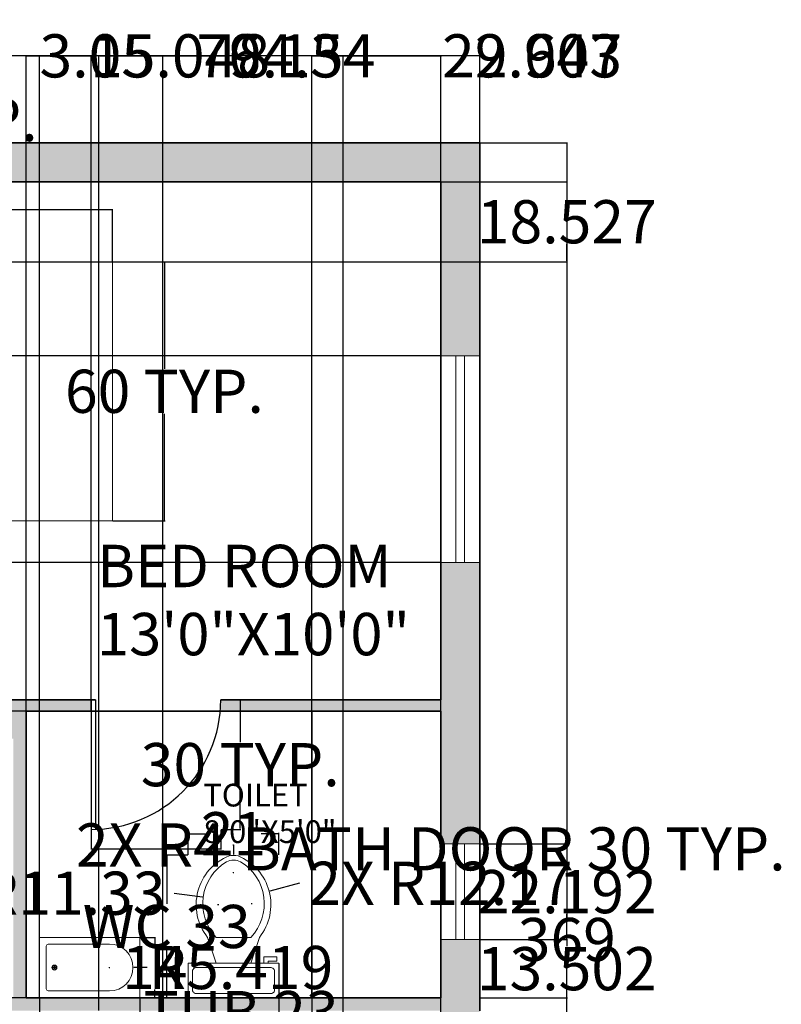
# Model space of a CAD drawing. Units: inches. Extents: x -75 to 484, y -248 to 214.
# Tile 7 of 7: x 308 to 484, y -52 to 176. Entities that reach past the tile are written whole.
import ezdxf

# ---------------------------------------------------------------- set-up
doc = ezdxf.new("R2010")
doc.units = ezdxf.units.IN
doc.header["$MEASUREMENT"] = 0
for name, color, linetype, lineweight in [('A-ANNO-DIMS', 2, 'Continuous', 18), ('A-AREA-IDEN', 7, 'Continuous', 18), ('A-DOOR', 3, 'Continuous', 25), ('A-FLOR-FIXT', 8, 'Continuous', 18), ('A-FURN', 8, 'Continuous', 18), ('A-GLAZ', 4, 'Continuous', 18), ('A-WALL', 7, 'Continuous', 35)]:
    doc.layers.add(name, color=color, linetype=linetype, lineweight=lineweight)
doc.layers.add('A-WALL-PATT', color=252, linetype='Continuous', lineweight=9, true_color=0x939598)
doc.styles.get("Standard").update_dxf_attribs({"font": 'arial.ttf'})
doc.dimstyles.get("Standard").update_dxf_attribs({"dimtxt": 10, "dimasz": 0.18, "dimexe": 0.18, "dimexo": 0.0625, "dimgap": 0.09, "dimtad": 0, "dimtih": 1, "dimtoh": 1, "dimdec": 0, "dimzin": 0, "dimdsep": 46, "dimlunit": 3, "dimtxsty": 'Standard', "dimcen": 0.09, "dimadec": 0, "dimazin": 0, "dimtfac": 1, "dimtdec": 0, "dimtofl": 0, "dimtmove": 0, "dimatfit": 3, "dimfxl": 1, "dimtolj": 1, "dimtzin": 0, "dimarcsym": 0})

# ---------------------------------------------------------------- blocks, each defined once
blk = doc.blocks.new('Bed - Queen')
for p, q in [((0, -80.00003), (0, 0)), ((0, 0), (59.99999, 0)), ((59.99999, 0), (59.99999, -80.00003)), ((7.99999, -1.2), (28.79998, -1.2)), ((7.99999, -14.4), (7.99999, -1.2)), ((28.79998, -1.2), (28.79998, -14.4)), ((31.19999, -1.2), (51.99999, -1.2)), ((31.19999, -14.4), (31.19999, -1.2)), ((51.99999, -1.2), (51.99999, -16.4)), ((0, -14.4), (44.8, -14.4)), ((59.99999, -29.6), (44.8, -14.4)), ((44.8, -14.4), (44.8, -29.6)), ((44.8, -16.8), (0, -16.8)), ((51.99999, -16.4), (46.79936, -16.4)), ((44.8, -29.6), (59.99999, -29.6)), ((59.99999, -80.00003), (0, -80.00003))]:
    blk.add_line(p, q)
blk = doc.blocks.new('Toilet - top')
for p, q in [((9.5, -6), (9.5, -2)), ((-10, -8.5), (-8, -8.5)), ((-10, -9.5), (-10, -8.5)), ((-8, -8.5), (-8, -8)), ((-7, -8), (-7, -9.5)), ((-4, -8), (-6, -14)), ((4, -8), (6, -14)), ((-7, -9.5), (-10, -9.5)), ((4, -14), (-4, -14))]:
    blk.add_line(p, q)
blk.add_lwpolyline([(10.5, -8), (10.5, 0), (-10.5, 0), (-10.5, -8)], close=True)
for points in [[(-9.5, -2), (-9.5, -6)], [(8.5, -1), (-8.5, -1)], [(-8.5, -7), (8.5, -7)]]:
    blk.add_lwpolyline(points)
for centre, radius, start, end in [((-8.62, -1.88), 0.884, 81.8699, 188.1301), ((8.62, -1.88), 0.884, 351.8699, 98.1301), ((-8.62, -6.12), 0.884, 171.8699, 278.1301), ((8.62, -6.12), 0.884, 261.8699, 8.1301), ((3.52, -21.58), 12.17, 141.4691, 247.9714), ((4.2, -21.82), 11.33, 136.3677, 238.9468), ((-3.52, -21.58), 12.17, 292.0284, 38.5307), ((-4.2, -21.82), 11.33, 301.053, 43.6321), ((0, -27.88), 4, 245.7318, 294.2682), ((0, -29), 4, 254.8605, 285.1395)]:
    blk.add_arc(centre, radius, start, end)
blk = doc.blocks.new('Bath Tub - 26 x 60 in.')
for p, q in [((9, -17), (9, -19)), ((8, -18), (10, -18))]:
    blk.add_line(p, q)
blk.add_lwpolyline([(0, -36), (0, 0), (60, 0), (60, -36)], close=True)
for points in [[(6, -4), (42, -4)], [(4, -30), (4, -6)], [(42, -32), (6, -32)]]:
    blk.add_lwpolyline(points)
for radius in [1.5, 1]:
    blk.add_circle((9, -18), radius)
for centre, radius, start, end in [((5.75, -5.75), 1.77, 81.8699, 188.1301), ((42, -18), 14, 270, 90), ((5.75, -30.25), 1.77, 171.8699, 278.1301)]:
    blk.add_arc(centre, radius, start, end)
blk = doc.blocks.new('DOOR-SINGLE-30')
for p, q in [((0, 30), (0, 0)), ((0, 30), (1, 30)), ((1, 30), (1, 0))]:
    blk.add_line(p, q)
blk.add_arc((0, 30), 30, 270, 0)
blk = doc.blocks.new('*D13')
at = {"layer": 'A-ANNO-DIMS', "color": 0, "lineweight": -2, "transparency": 16777216}
for p, q in [((184.9, 147.72), (184.9, 153.24)), ((185.08, 153.06), (220.72, 153.06)), ((220.9, 147.72), (220.9, 153.24)), ((220.9, 153.06), (221.08, 153.06))]:
    blk.add_line(p, q, dxfattribs=at)
at = {"layer": 'A-ANNO-DIMS', "color": 0, "transparency": 16777216}
for points in [[(185.08, 153.09), (185.08, 153.03), (184.9, 153.06)], [(220.72, 153.09), (220.72, 153.03), (220.9, 153.06)]]:
    blk.add_solid(points, dxfattribs=at)
at = {"layer": 'Defpoints', "color": 0, "transparency": 16777216}
for p in [(220.9, 153.06), (184.9, 147.66), (220.9, 147.66)]:
    blk.add_point(p, dxfattribs=at)
at = {"layer": 'A-ANNO-DIMS', "color": 0, "transparency": 16777216, "insert": (268.16, 153.06), "char_height": 10, "attachment_point": 5}
blk.add_mtext('\\A1;DOOR 36 TYP.', dxfattribs=at)
blk = doc.blocks.new('*D15')
at = {"layer": 'A-ANNO-DIMS', "color": 0, "lineweight": -2, "transparency": 16777216}
for p, q in [((324.26, -11.41), (324.26, -16.02)), ((354.26, -11.41), (354.26, -16.02)), ((324.44, -15.84), (354.08, -15.84)), ((354.26, -15.84), (354.44, -15.84))]:
    blk.add_line(p, q, dxfattribs=at)
at = {"layer": 'A-ANNO-DIMS', "color": 0, "transparency": 16777216}
for points in [[(324.44, -15.81), (324.44, -15.87), (324.26, -15.84)], [(354.08, -15.81), (354.08, -15.87), (354.26, -15.84)]]:
    blk.add_solid(points, dxfattribs=at)
at = {"layer": 'Defpoints', "color": 0, "transparency": 16777216}
for p in [(324.26, -11.34), (354.26, -11.34), (354.26, -15.84)]:
    blk.add_point(p, dxfattribs=at)
at = {"layer": 'A-ANNO-DIMS', "color": 0, "transparency": 16777216, "insert": (422.11, -15.84), "char_height": 10, "attachment_point": 5}
blk.add_mtext('\\A1;BATH DOOR 30 TYP.', dxfattribs=at)
blk = doc.blocks.new('*D16')
at = {"layer": 'A-ANNO-DIMS', "color": 0, "lineweight": -2, "transparency": 16777216}
for p, q in [((354.32, 18.66), (358.94, 18.66)), ((358.76, 18.48), (358.76, 8.86)), ((358.76, -11.16), (358.76, -1.54)), ((354.32, -11.34), (358.94, -11.34))]:
    blk.add_line(p, q, dxfattribs=at)
at = {"layer": 'A-ANNO-DIMS', "color": 0, "transparency": 16777216}
for points in [[(358.73, 18.48), (358.79, 18.48), (358.76, 18.66)], [(358.73, -11.16), (358.79, -11.16), (358.76, -11.34)]]:
    blk.add_solid(points, dxfattribs=at)
at = {"layer": 'Defpoints', "color": 0, "transparency": 16777216}
for p in [(354.26, 18.66), (358.76, 18.66), (354.26, -11.34)]:
    blk.add_point(p, dxfattribs=at)
at = {"layer": 'A-ANNO-DIMS', "color": 0, "transparency": 16777216, "insert": (358.76, 3.66), "char_height": 10, "attachment_point": 5}
blk.add_mtext('\\A1;30 TYP.', dxfattribs=at)
blk = doc.blocks.new('*D19')
at = {"layer": 'A-ANNO-DIMS', "color": 0, "lineweight": -2, "transparency": 16777216}
for p, q in [((249.21, 120.19), (249.21, 132.31)), ((329.21, 120.19), (329.21, 132.31)), ((249.21, 132.13), (249.03, 132.13)), ((329.03, 132.13), (249.39, 132.13))]:
    blk.add_line(p, q, dxfattribs=at)
at = {"layer": 'A-ANNO-DIMS', "color": 0, "transparency": 16777216}
for points in [[(249.39, 132.16), (249.39, 132.1), (249.21, 132.13)], [(329.03, 132.16), (329.03, 132.1), (329.21, 132.13)]]:
    blk.add_solid(points, dxfattribs=at)
at = {"layer": 'Defpoints', "color": 0, "transparency": 16777216}
for p in [(249.21, 132.13), (249.21, 120.13), (329.21, 120.13)]:
    blk.add_point(p, dxfattribs=at)
at = {"layer": 'A-ANNO-DIMS', "color": 0, "transparency": 16777216, "insert": (181.53, 132.13), "char_height": 10, "attachment_point": 5}
blk.add_mtext('\\A1;QUEEN BED 80 TYP.', dxfattribs=at)
blk = doc.blocks.new('*D20')
at = {"layer": 'A-ANNO-DIMS', "color": 0, "lineweight": -2, "transparency": 16777216}
for p, q in [((329.27, 120.13), (341.39, 120.13)), ((341.21, 119.95), (341.21, 95.33)), ((341.21, 60.31), (341.21, 84.93)), ((329.27, 60.13), (341.39, 60.13))]:
    blk.add_line(p, q, dxfattribs=at)
at = {"layer": 'A-ANNO-DIMS', "color": 0, "transparency": 16777216}
for points in [[(341.18, 119.95), (341.24, 119.95), (341.21, 120.13)], [(341.18, 60.31), (341.24, 60.31), (341.21, 60.13)]]:
    blk.add_solid(points, dxfattribs=at)
at = {"layer": 'Defpoints', "color": 0, "transparency": 16777216}
for p in [(329.21, 120.13), (341.21, 120.13), (329.21, 60.13)]:
    blk.add_point(p, dxfattribs=at)
at = {"layer": 'A-ANNO-DIMS', "color": 0, "transparency": 16777216, "insert": (341.21, 90.13), "char_height": 10, "attachment_point": 5}
blk.add_mtext('\\A1;60 TYP.', dxfattribs=at)
blk = doc.blocks.new('*D31')
at = {"layer": 'A-ANNO-DIMS', "color": 0, "lineweight": -2, "transparency": 16777216}
for p, q in [((346.65, -17.3), (341.57, -17.3)), ((341.75, -17.48), (341.75, -28.56)), ((341.75, -50.16), (341.75, -39.08)), ((346.65, -50.34), (341.57, -50.34))]:
    blk.add_line(p, q, dxfattribs=at)
at = {"layer": 'A-ANNO-DIMS', "color": 0, "transparency": 16777216}
for points in [[(341.72, -17.48), (341.78, -17.48), (341.75, -17.3)], [(341.72, -50.16), (341.78, -50.16), (341.75, -50.34)]]:
    blk.add_solid(points, dxfattribs=at)
at = {"layer": 'Defpoints', "color": 0, "transparency": 16777216}
for p in [(346.71, -17.3), (341.75, -50.34), (346.71, -50.34)]:
    blk.add_point(p, dxfattribs=at)
at = {"layer": 'A-ANNO-DIMS', "color": 0, "transparency": 16777216, "insert": (341.75, -33.82), "char_height": 10, "attachment_point": 5}
blk.add_mtext('\\A1;WC 33', dxfattribs=at)
blk = doc.blocks.new('*D32')
at = {"layer": 'A-ANNO-DIMS', "color": 0, "lineweight": -2, "transparency": 16777216}
for p, q in [((346.71, -17.23), (346.71, -12.16)), ((346.89, -12.34), (350.84, -12.34)), ((367.53, -12.34), (363.58, -12.34)), ((367.71, -17.23), (367.71, -12.16))]:
    blk.add_line(p, q, dxfattribs=at)
at = {"layer": 'A-ANNO-DIMS', "color": 0, "transparency": 16777216}
for points in [[(346.89, -12.31), (346.89, -12.37), (346.71, -12.34)], [(367.53, -12.31), (367.53, -12.37), (367.71, -12.34)]]:
    blk.add_solid(points, dxfattribs=at)
at = {"layer": 'Defpoints', "color": 0, "transparency": 16777216}
for p in [(346.71, -12.34), (346.71, -17.3), (367.71, -17.3)]:
    blk.add_point(p, dxfattribs=at)
at = {"layer": 'A-ANNO-DIMS', "color": 0, "transparency": 16777216, "insert": (357.21, -12.34), "char_height": 10, "attachment_point": 5}
blk.add_mtext('\\A1;21', dxfattribs=at)
blk = doc.blocks.new('*D35')
at = {"layer": 'A-ANNO-DIMS', "color": 0, "lineweight": -2, "transparency": 16777216}
for p, q in [((312.26, -50.35), (312.26, -53.95)), ((335.49, -50.35), (335.49, -53.95)), ((312.44, -53.77), (335.31, -53.77)), ((335.49, -53.77), (335.67, -53.77))]:
    blk.add_line(p, q, dxfattribs=at)
at = {"layer": 'A-ANNO-DIMS', "color": 0, "transparency": 16777216}
for points in [[(312.44, -53.74), (312.44, -53.8), (312.26, -53.77)], [(335.31, -53.74), (335.31, -53.8), (335.49, -53.77)]]:
    blk.add_solid(points, dxfattribs=at)
at = {"layer": 'Defpoints', "color": 0, "transparency": 16777216}
for p in [(312.26, -50.29), (335.49, -50.29), (335.49, -53.77)]:
    blk.add_point(p, dxfattribs=at)
at = {"layer": 'A-ANNO-DIMS', "color": 0, "transparency": 16777216, "insert": (358.96, -53.77), "char_height": 10, "attachment_point": 5}
blk.add_mtext('\\A1;TUB 23', dxfattribs=at)
blk = doc.blocks.new('*D36')
at = {"layer": 'A-ANNO-DIMS', "color": 0, "lineweight": -2, "transparency": 16777216}
for p, q in [((335.55, -36.35), (339.15, -36.35)), ((338.97, -36.53), (338.97, -38.21)), ((338.97, -50.11), (338.97, -48.43)), ((335.55, -50.29), (339.15, -50.29))]:
    blk.add_line(p, q, dxfattribs=at)
at = {"layer": 'A-ANNO-DIMS', "color": 0, "transparency": 16777216}
for points in [[(338.94, -36.53), (339, -36.53), (338.97, -36.35)], [(338.94, -50.11), (339, -50.11), (338.97, -50.29)]]:
    blk.add_solid(points, dxfattribs=at)
at = {"layer": 'Defpoints', "color": 0, "transparency": 16777216}
for p in [(335.49, -36.35), (338.97, -36.35), (335.49, -50.29)]:
    blk.add_point(p, dxfattribs=at)
at = {"layer": 'A-ANNO-DIMS', "color": 0, "transparency": 16777216, "insert": (338.97, -43.32), "char_height": 10, "attachment_point": 5}
blk.add_mtext('\\A1;14', dxfattribs=at)
blk = doc.blocks.new('*D41')
at = {"layer": 'A-ANNO-DIMS', "color": 0, "lineweight": -2, "transparency": 16777216}
for p, q in [((15.21, 147.72), (15.21, 167.99)), ((15.39, 167.81), (203.57, 167.81)), ((414.03, 167.81), (225.85, 167.81)), ((414.21, 147.72), (414.21, 167.99))]:
    blk.add_line(p, q, dxfattribs=at)
at = {"layer": 'A-ANNO-DIMS', "color": 0, "transparency": 16777216}
for points in [[(15.39, 167.84), (15.39, 167.78), (15.21, 167.81)], [(414.03, 167.84), (414.03, 167.78), (414.21, 167.81)]]:
    blk.add_solid(points, dxfattribs=at)
at = {"layer": 'Defpoints', "color": 0, "transparency": 16777216}
for p in [(414.21, 167.81), (15.21, 147.66), (414.21, 147.66)]:
    blk.add_point(p, dxfattribs=at)
at = {"layer": 'A-ANNO-DIMS', "color": 0, "transparency": 16777216, "insert": (214.71, 167.81), "char_height": 10, "attachment_point": 5}
blk.add_mtext('\\A1;399', dxfattribs=at)
blk = doc.blocks.new('*D42')
at = {"layer": 'A-ANNO-DIMS', "color": 0, "lineweight": -2, "transparency": 16777216}
for p, q in [((414.27, 147.66), (434.54, 147.66)), ((434.36, 147.48), (434.36, -31.64)), ((434.36, -221.16), (434.36, -42.04)), ((414.27, -221.34), (434.54, -221.34))]:
    blk.add_line(p, q, dxfattribs=at)
at = {"layer": 'A-ANNO-DIMS', "color": 0, "transparency": 16777216}
for points in [[(434.33, 147.48), (434.39, 147.48), (434.36, 147.66)], [(434.33, -221.16), (434.39, -221.16), (434.36, -221.34)]]:
    blk.add_solid(points, dxfattribs=at)
at = {"layer": 'Defpoints', "color": 0, "transparency": 16777216}
for p in [(414.21, 147.66), (414.21, -221.34), (434.36, -221.34)]:
    blk.add_point(p, dxfattribs=at)
at = {"layer": 'A-ANNO-DIMS', "color": 0, "transparency": 16777216, "insert": (434.36, -36.84), "char_height": 10, "attachment_point": 5}
blk.add_mtext('\\A1;369', dxfattribs=at)
blk = doc.blocks.new('*D50')
at = {"layer": 'A-ANNO-DIMS', "color": 0, "lineweight": -2, "transparency": 16777216}
for p, q in [((405.15, 138.66), (-5.12, 138.66)), ((-4.94, 138.48), (-4.94, 123.68)), ((-4.94, 98.48), (-4.94, 113.28)), ((405.15, 98.3), (-5.12, 98.3))]:
    blk.add_line(p, q, dxfattribs=at)
at = {"layer": 'A-ANNO-DIMS', "color": 0, "transparency": 16777216}
for points in [[(-4.97, 138.48), (-4.91, 138.48), (-4.94, 138.66)], [(-4.97, 98.48), (-4.91, 98.48), (-4.94, 98.3)]]:
    blk.add_solid(points, dxfattribs=at)
at = {"layer": 'Defpoints', "color": 0, "transparency": 16777216}
for p in [(405.21, 138.66), (-4.94, 98.3), (405.21, 98.3)]:
    blk.add_point(p, dxfattribs=at)
at = {"layer": 'A-ANNO-DIMS', "color": 0, "transparency": 16777216, "insert": (-4.94, 118.48), "char_height": 10, "attachment_point": 5}
blk.add_mtext('\\A1;40.35', dxfattribs=at)
blk = doc.blocks.new('*D51')
at = {"layer": 'A-ANNO-DIMS', "color": 0, "lineweight": -2, "transparency": 16777216}
for p, q in [((405.15, 98.3), (-5.12, 98.3)), ((-4.94, 98.12), (-4.94, 79.59)), ((-4.94, 50.66), (-4.94, 69.2)), ((405.15, 50.48), (-5.12, 50.48))]:
    blk.add_line(p, q, dxfattribs=at)
at = {"layer": 'A-ANNO-DIMS', "color": 0, "transparency": 16777216}
for points in [[(-4.97, 98.12), (-4.91, 98.12), (-4.94, 98.3)], [(-4.97, 50.66), (-4.91, 50.66), (-4.94, 50.48)]]:
    blk.add_solid(points, dxfattribs=at)
at = {"layer": 'Defpoints', "color": 0, "transparency": 16777216}
for p in [(405.21, 98.3), (-4.94, 50.48), (405.21, 50.48)]:
    blk.add_point(p, dxfattribs=at)
at = {"layer": 'A-ANNO-DIMS', "color": 0, "transparency": 16777216, "insert": (-4.94, 74.39), "char_height": 10, "attachment_point": 5}
blk.add_mtext('\\A1;47.82', dxfattribs=at)
blk = doc.blocks.new('*D52')
at = {"layer": 'A-ANNO-DIMS', "color": 0, "lineweight": -2, "transparency": 16777216}
for p, q in [((414.27, -36.84), (434.54, -36.84)), ((434.36, -37.02), (434.36, -38.39)), ((434.36, -50.16), (434.36, -48.79)), ((414.27, -50.34), (434.54, -50.34))]:
    blk.add_line(p, q, dxfattribs=at)
at = {"layer": 'A-ANNO-DIMS', "color": 0, "transparency": 16777216}
for points in [[(434.33, -37.02), (434.39, -37.02), (434.36, -36.84)], [(434.33, -50.16), (434.39, -50.16), (434.36, -50.34)]]:
    blk.add_solid(points, dxfattribs=at)
at = {"layer": 'Defpoints', "color": 0, "transparency": 16777216}
for p in [(414.21, -36.84), (434.36, -36.84), (414.21, -50.34)]:
    blk.add_point(p, dxfattribs=at)
at = {"layer": 'A-ANNO-DIMS', "color": 0, "transparency": 16777216, "insert": (434.36, -43.59), "char_height": 10, "attachment_point": 5}
blk.add_mtext('\\A1;13.502', dxfattribs=at)
blk = doc.blocks.new('*D53')
at = {"layer": 'A-ANNO-DIMS', "color": 0, "lineweight": -2, "transparency": 16777216}
for p, q in [((414.27, -14.65), (434.54, -14.65)), ((434.36, -14.83), (434.36, -20.55)), ((434.36, -36.66), (434.36, -30.94)), ((414.27, -36.84), (434.54, -36.84))]:
    blk.add_line(p, q, dxfattribs=at)
at = {"layer": 'A-ANNO-DIMS', "color": 0, "transparency": 16777216}
for points in [[(434.33, -14.83), (434.39, -14.83), (434.36, -14.65)], [(434.33, -36.66), (434.39, -36.66), (434.36, -36.84)]]:
    blk.add_solid(points, dxfattribs=at)
at = {"layer": 'Defpoints', "color": 0, "transparency": 16777216}
for p in [(414.21, -14.65), (414.21, -36.84), (434.36, -36.84)]:
    blk.add_point(p, dxfattribs=at)
at = {"layer": 'A-ANNO-DIMS', "color": 0, "transparency": 16777216, "insert": (434.36, -25.75), "char_height": 10, "attachment_point": 5}
blk.add_mtext('\\A1;22.192', dxfattribs=at)
blk = doc.blocks.new('*D59')
at = {"layer": 'A-ANNO-DIMS', "color": 0, "lineweight": -2, "transparency": 16777216}
for p, q in [((309.21, 16.11), (309.21, 167.99)), ((309.39, 167.81), (324.08, 167.81)), ((324.26, 16.11), (324.26, 167.99)), ((324.26, 167.81), (324.44, 167.81))]:
    blk.add_line(p, q, dxfattribs=at)
at = {"layer": 'A-ANNO-DIMS', "color": 0, "transparency": 16777216}
for points in [[(309.39, 167.84), (309.39, 167.78), (309.21, 167.81)], [(324.08, 167.84), (324.08, 167.78), (324.26, 167.81)]]:
    blk.add_solid(points, dxfattribs=at)
at = {"layer": 'Defpoints', "color": 0, "transparency": 16777216}
for p in [(324.26, 167.81), (309.21, 16.05), (324.26, 16.05)]:
    blk.add_point(p, dxfattribs=at)
at = {"layer": 'A-ANNO-DIMS', "color": 0, "transparency": 16777216, "insert": (344.82, 167.81), "char_height": 10, "attachment_point": 5}
blk.add_mtext('\\A1;15.048', dxfattribs=at)
blk = doc.blocks.new('*D60')
at = {"layer": 'A-ANNO-DIMS', "color": 0, "lineweight": -2, "transparency": 16777216}
for p, q in [((375.24, 16.05), (-5.12, 16.05)), ((-4.94, 15.87), (-4.94, -11.95)), ((-4.94, -50.16), (-4.94, -22.35)), ((375.24, -50.34), (-5.12, -50.34))]:
    blk.add_line(p, q, dxfattribs=at)
at = {"layer": 'A-ANNO-DIMS', "color": 0, "transparency": 16777216}
for points in [[(-4.97, 15.87), (-4.91, 15.87), (-4.94, 16.05)], [(-4.97, -50.16), (-4.91, -50.16), (-4.94, -50.34)]]:
    blk.add_solid(points, dxfattribs=at)
at = {"layer": 'Defpoints', "color": 0, "transparency": 16777216}
for p in [(375.3, 16.05), (-4.94, -50.34), (375.3, -50.34)]:
    blk.add_point(p, dxfattribs=at)
at = {"layer": 'A-ANNO-DIMS', "color": 0, "transparency": 16777216, "insert": (-4.94, -17.15), "char_height": 10, "attachment_point": 5}
blk.add_mtext('\\A1;66.39', dxfattribs=at)
blk = doc.blocks.new('*D61')
at = {"layer": 'A-ANNO-DIMS', "color": 0, "lineweight": -2, "transparency": 16777216}
for p, q in [((375.3, 16.11), (375.3, 167.99)), ((375.48, 167.81), (405.03, 167.81)), ((405.21, 16.11), (405.21, 167.99)), ((405.21, 167.81), (405.39, 167.81))]:
    blk.add_line(p, q, dxfattribs=at)
at = {"layer": 'A-ANNO-DIMS', "color": 0, "transparency": 16777216}
for points in [[(375.48, 167.84), (375.48, 167.78), (375.3, 167.81)], [(405.03, 167.84), (405.03, 167.78), (405.21, 167.81)]]:
    blk.add_solid(points, dxfattribs=at)
at = {"layer": 'Defpoints', "color": 0, "transparency": 16777216}
for p in [(405.21, 167.81), (375.3, 16.05), (405.21, 16.05)]:
    blk.add_point(p, dxfattribs=at)
at = {"layer": 'A-ANNO-DIMS', "color": 0, "transparency": 16777216, "insert": (426.32, 167.81), "char_height": 10, "attachment_point": 5}
blk.add_mtext('\\A1;29.907', dxfattribs=at)
blk = doc.blocks.new('*D64')
at = {"layer": 'A-ANNO-DIMS', "color": 0, "lineweight": -2, "transparency": 16777216}
for p, q in [((326.06, -53.28), (326.06, 167.99)), ((326.24, 167.81), (348.67, 167.81)), ((405.03, 167.81), (382.59, 167.81)), ((405.21, -53.28), (405.21, 167.99))]:
    blk.add_line(p, q, dxfattribs=at)
at = {"layer": 'A-ANNO-DIMS', "color": 0, "transparency": 16777216}
for points in [[(326.24, 167.84), (326.24, 167.78), (326.06, 167.81)], [(405.03, 167.84), (405.03, 167.78), (405.21, 167.81)]]:
    blk.add_solid(points, dxfattribs=at)
at = {"layer": 'Defpoints', "color": 0, "transparency": 16777216}
for p in [(405.21, 167.81), (326.06, -53.34), (405.21, -53.34)]:
    blk.add_point(p, dxfattribs=at)
at = {"layer": 'A-ANNO-DIMS', "color": 0, "transparency": 16777216, "insert": (365.63, 167.81), "char_height": 10, "attachment_point": 5}
blk.add_mtext('\\A1;79.15', dxfattribs=at)
blk = doc.blocks.new('*D65')
at = {"layer": 'A-ANNO-DIMS', "color": 0, "lineweight": -2, "transparency": 16777216}
for p, q in [((340.87, -142.28), (340.87, 167.99)), ((341.05, 167.81), (356.07, 167.81)), ((405.03, 167.81), (390.01, 167.81)), ((405.21, -142.28), (405.21, 167.99))]:
    blk.add_line(p, q, dxfattribs=at)
at = {"layer": 'A-ANNO-DIMS', "color": 0, "transparency": 16777216}
for points in [[(341.05, 167.84), (341.05, 167.78), (340.87, 167.81)], [(405.03, 167.84), (405.03, 167.78), (405.21, 167.81)]]:
    blk.add_solid(points, dxfattribs=at)
at = {"layer": 'Defpoints', "color": 0, "transparency": 16777216}
for p in [(405.21, 167.81), (340.87, -142.34), (405.21, -142.34)]:
    blk.add_point(p, dxfattribs=at)
at = {"layer": 'A-ANNO-DIMS', "color": 0, "transparency": 16777216, "insert": (373.04, 167.81), "char_height": 10, "attachment_point": 5}
blk.add_mtext('\\A1;64.34', dxfattribs=at)
blk = doc.blocks.new('*D66')
at = {"layer": 'A-ANNO-DIMS', "color": 0, "lineweight": -2, "transparency": 16777216}
for p, q in [((382.57, -85.27), (382.57, 167.99)), ((382.75, 167.81), (405.03, 167.81)), ((405.21, -85.27), (405.21, 167.99)), ((405.21, 167.81), (405.39, 167.81))]:
    blk.add_line(p, q, dxfattribs=at)
at = {"layer": 'A-ANNO-DIMS', "color": 0, "transparency": 16777216}
for points in [[(382.75, 167.84), (382.75, 167.78), (382.57, 167.81)], [(405.03, 167.84), (405.03, 167.78), (405.21, 167.81)]]:
    blk.add_solid(points, dxfattribs=at)
at = {"layer": 'Defpoints', "color": 0, "transparency": 16777216}
for p in [(405.21, 167.81), (382.57, -85.33), (405.21, -85.33)]:
    blk.add_point(p, dxfattribs=at)
at = {"layer": 'A-ANNO-DIMS', "color": 0, "transparency": 16777216, "insert": (426.32, 167.81), "char_height": 10, "attachment_point": 5}
blk.add_mtext('\\A1;22.643', dxfattribs=at)
blk = doc.blocks.new('*D75')
at = {"layer": 'A-ANNO-DIMS', "color": 0, "lineweight": -2, "transparency": 16777216}
for p, q in [((249.27, 138.66), (434.54, 138.66)), ((434.36, 138.48), (434.36, 134.59)), ((434.36, 120.31), (434.36, 124.2)), ((249.27, 120.13), (434.54, 120.13))]:
    blk.add_line(p, q, dxfattribs=at)
at = {"layer": 'A-ANNO-DIMS', "color": 0, "transparency": 16777216}
for points in [[(434.33, 138.48), (434.39, 138.48), (434.36, 138.66)], [(434.33, 120.31), (434.39, 120.31), (434.36, 120.13)]]:
    blk.add_solid(points, dxfattribs=at)
at = {"layer": 'Defpoints', "color": 0, "transparency": 16777216}
for p in [(249.21, 138.66), (249.21, 120.13), (434.36, 120.13)]:
    blk.add_point(p, dxfattribs=at)
at = {"layer": 'A-ANNO-DIMS', "color": 0, "transparency": 16777216, "insert": (434.36, 129.39), "char_height": 10, "attachment_point": 5}
blk.add_mtext('\\A1;18.527', dxfattribs=at)
blk = doc.blocks.new('*D79')
at = {"layer": 'A-ANNO-DIMS', "color": 0, "lineweight": -2, "transparency": 16777216}
for p, q in [((309.21, -50.28), (309.21, 167.99)), ((309.39, 167.81), (312.08, 167.81)), ((312.26, -50.23), (312.26, 167.99)), ((312.26, 167.81), (312.44, 167.81))]:
    blk.add_line(p, q, dxfattribs=at)
at = {"layer": 'A-ANNO-DIMS', "color": 0, "transparency": 16777216}
for points in [[(309.39, 167.84), (309.39, 167.78), (309.21, 167.81)], [(312.08, 167.84), (312.08, 167.78), (312.26, 167.81)]]:
    blk.add_solid(points, dxfattribs=at)
at = {"layer": 'Defpoints', "color": 0, "transparency": 16777216}
for p in [(312.26, 167.81), (309.21, -50.34), (312.26, -50.29)]:
    blk.add_point(p, dxfattribs=at)
at = {"layer": 'A-ANNO-DIMS', "color": 0, "transparency": 16777216, "insert": (325.55, 167.81), "char_height": 10, "attachment_point": 5}
blk.add_mtext('\\A1;3.05', dxfattribs=at)
blk = doc.blocks.new('*D80')
at = {"layer": 'A-ANNO-DIMS', "color": 0, "lineweight": -2, "transparency": 16777216}
for p, q in [((367.71, -42.41), (367.71, -241.67)), ((375.3, -50.41), (375.3, -241.67)), ((367.89, -241.49), (375.12, -241.49)), ((375.3, -241.49), (375.48, -241.49))]:
    blk.add_line(p, q, dxfattribs=at)
at = {"layer": 'A-ANNO-DIMS', "color": 0, "transparency": 16777216}
for points in [[(367.89, -241.46), (367.89, -241.52), (367.71, -241.49)], [(375.12, -241.46), (375.12, -241.52), (375.3, -241.49)]]:
    blk.add_solid(points, dxfattribs=at)
at = {"layer": 'Defpoints', "color": 0, "transparency": 16777216}
for p in [(367.71, -42.34), (375.3, -50.34), (375.3, -241.49)]:
    blk.add_point(p, dxfattribs=at)
at = {"layer": 'A-ANNO-DIMS', "color": 0, "transparency": 16777216, "insert": (392.4, -241.49), "char_height": 10, "attachment_point": 5}
blk.add_mtext('\\A1;7.593', dxfattribs=at)
blk = doc.blocks.new('*D90')
at = {"layer": 'A-ANNO-DIMS', "color": 0, "lineweight": -2, "transparency": 16777216}
for p, q in [((372.52, -23.82), (365.63, -25.63)), ((353.6, -28.76), (353.78, -28.76)), ((353.69, -28.85), (353.69, -28.67))]:
    blk.add_line(p, q, dxfattribs=at)
at = {"layer": 'A-ANNO-DIMS', "color": 0, "transparency": 16777216}
blk.add_solid([(365.63, -25.6), (365.64, -25.65), (365.46, -25.67)], dxfattribs=at)
at = {"layer": 'Defpoints', "color": 0, "transparency": 16777216}
for p in [(365.46, -25.67), (353.69, -28.76)]:
    blk.add_point(p, dxfattribs=at)
at = {"layer": 'A-ANNO-DIMS', "color": 0, "transparency": 16777216, "insert": (405.1, -23.82), "char_height": 10, "attachment_point": 5}
blk.add_mtext('\\A1;2X R12.17', dxfattribs=at)
blk = doc.blocks.new('*D91')
at = {"layer": 'A-ANNO-DIMS', "color": 0, "lineweight": -2, "transparency": 16777216}
for p, q in [((343.44, -26.11), (350, -26.99)), ((361.32, -28.53), (361.5, -28.53)), ((361.41, -28.62), (361.41, -28.44))]:
    blk.add_line(p, q, dxfattribs=at)
at = {"layer": 'A-ANNO-DIMS', "color": 0, "transparency": 16777216}
blk.add_solid([(350.01, -26.96), (350, -27.02), (350.18, -27.02)], dxfattribs=at)
at = {"layer": 'Defpoints', "color": 0, "transparency": 16777216}
for p in [(350.18, -27.02), (361.41, -28.53)]:
    blk.add_point(p, dxfattribs=at)
at = {"layer": 'A-ANNO-DIMS', "color": 0, "transparency": 16777216, "insert": (310.87, -26.11), "char_height": 10, "attachment_point": 5}
blk.add_mtext('\\A1;2X R11.33', dxfattribs=at)
blk = doc.blocks.new('*D92')
at = {"layer": 'A-ANNO-DIMS', "color": 0, "lineweight": -2, "transparency": 16777216}
for p, q in [((357.03, -14.94), (357.21, -14.94)), ((357.21, -14.94), (357.21, -17.16)), ((357.12, -21.34), (357.3, -21.34)), ((357.21, -21.43), (357.21, -21.25))]:
    blk.add_line(p, q, dxfattribs=at)
at = {"layer": 'A-ANNO-DIMS', "color": 0, "transparency": 16777216}
blk.add_solid([(357.24, -17.16), (357.18, -17.16), (357.21, -17.34)], dxfattribs=at)
at = {"layer": 'Defpoints', "color": 0, "transparency": 16777216}
for p in [(357.21, -17.34), (357.21, -21.34)]:
    blk.add_point(p, dxfattribs=at)
at = {"layer": 'A-ANNO-DIMS', "color": 0, "transparency": 16777216, "insert": (338.07, -14.94), "char_height": 10, "attachment_point": 5}
blk.add_mtext('\\A1;2X R4', dxfattribs=at)
blk = doc.blocks.new('*D93')
at = {"layer": 'A-ANNO-DIMS', "color": 0, "lineweight": -2, "transparency": 16777216}
for p, q in [((328.43, -43.32), (328.61, -43.32)), ((328.52, -43.41), (328.52, -43.23)), ((337.19, -43.32), (334.12, -43.32))]:
    blk.add_line(p, q, dxfattribs=at)
at = {"layer": 'A-ANNO-DIMS', "color": 0, "transparency": 16777216}
blk.add_solid([(334.12, -43.29), (334.12, -43.35), (333.94, -43.32)], dxfattribs=at)
at = {"layer": 'Defpoints', "color": 0, "transparency": 16777216}
for p in [(328.52, -43.32), (333.94, -43.32)]:
    blk.add_point(p, dxfattribs=at)
at = {"layer": 'A-ANNO-DIMS', "color": 0, "transparency": 16777216, "insert": (358.95, -43.32), "char_height": 10, "attachment_point": 5}
blk.add_mtext('\\A1;R5.419', dxfattribs=at)

msp = doc.modelspace()

# ---------------------------------------------------------------- hatches: boundary and pattern name
at = {"layer": 'A-WALL-PATT'}
h = msp.add_hatch(color=256, dxfattribs=at)
h.dxf.hatch_style = 1
h.paths.add_polyline_path([(184.9004, 147.6567), (15.2094, 147.6567), (15.2094, 92.5031), (24.2094, 92.5031), (24.2094, 138.6567), (186.0436, 138.6567, -0.06325422)])
h.paths.add_polyline_path([(414.2094, 147.6567), (249.2094, 147.6567), (220.9004, 147.6567), (220.9004, 138.6567), (240.2094, 138.6567), (240.2094, 18.6567), (240.2094, 9.6567), (249.2094, 9.6567), (249.2094, 45.6567), (249.2094, 138.6567), (405.2094, 138.6567), (405.2094, 98.3029), (414.2094, 98.3029)])
h.paths.add_polyline_path([(159.2094, 18.6567), (24.2094, 18.6567), (24.2094, 44.5861), (15.2094, 44.5861), (15.2094, 9.6567), (15.2094, -3.1791), (24.2094, -3.1791), (24.2094, 9.6567), (132.2094, 9.6567), (132.2094, -50.3433), (83.7394, -50.3433), (83.7394, -53.3433), (132.2094, -53.3433), (159.2094, -53.3433), (159.2094, -50.3433), (135.2094, -50.3433), (135.2094, 9.6567), (159.2094, 9.6567)])
h.paths.add_polyline_path([(53.8898, -50.3433), (24.2094, -50.3433), (24.2094, -27.303), (15.2094, -27.303), (15.2094, -50.3433), (15.2094, -53.3433), (15.2094, -74.0487), (24.2094, -74.0487), (24.2094, -53.3433), (53.7394, -53.3433, -0.02504709)])
h.paths.add_polyline_path([(24.2094, -121.9657), (15.2094, -121.9657), (15.2094, -212.3433), (15.2094, -221.3433), (24.2094, -221.3433), (84.3017, -221.3433), (84.3017, -212.3433), (24.2094, -212.3433)])
h.paths.add_polyline_path([(414.2094, -155.3433), (414.2094, -53.3433), (414.2094, -50.3433), (414.2094, -36.8417), (405.2094, -36.8417), (405.2094, -50.3433), (309.2094, -50.3433), (309.2094, 16.0463), (324.2573, 16.0463), (324.2573, 18.6567), (284.0663, 18.6567, -0.06325422), (285.2094, 9.6567), (306.2094, 9.6567), (306.2094, -50.3433), (285.2094, -50.3433), (285.2094, -53.3433), (309.2094, -53.3433), (405.2094, -53.3433), (405.2094, -212.3433), (293.2094, -212.3433), (293.2094, -158.3433), (293.2094, -145.3433), (300.0339, -145.3433), (300.0339, -142.3433), (285.2094, -142.3433), (159.2094, -142.3433), (159.2094, -89.3433, -0.02086055), (156.2094, -89.218), (156.2094, -212.3433), (131.9001, -212.3433), (131.9001, -221.3433), (156.2094, -221.3433), (165.2094, -221.3433), (285.2094, -221.3433), (288.6713, -221.3433), (293.2094, -221.3433), (405.2094, -221.3433), (414.2094, -221.3433)])
h.paths.add_polyline_path([(165.2094, -212.3433), (165.2094, -151.3433), (285.2094, -151.3433), (285.2094, -212.3433)], flags=16)
h.paths.add_polyline_path([(189.462, -195.5437), (182.159, -190.2838, -0.23606798), (182.5164, -188.0765), (181.7049, -187.4921), (185.5037, -182.2177), (184.648, -181.6013, -0.04492589), (180.0821, -186.3232), (179.2706, -185.7388), (189.206, -171.9443), (190.0174, -172.5287, -0.04492589), (186.9857, -178.3556), (187.8415, -178.9719), (191.6403, -173.6976), (192.4517, -174.282, -0.23606798), (194.432, -173.2435), (201.735, -178.5034, -0.23606798), (201.3776, -180.7107), (202.189, -181.2952, -0.11764706), (192.2537, -195.0897), (191.4423, -194.5053, -0.23606798)], flags=0)
h.paths.add_polyline_path([(253.751, -177.9543), (254.5293, -177.3263, -0.23606798), (254.0517, -175.1419), (261.056, -169.4904, -0.23606798), (263.0902, -170.419), (263.8684, -169.7911), (267.95, -174.8498), (268.7708, -174.1875, -0.04492589), (265.425, -168.5352), (266.2032, -167.9073), (276.8782, -181.1378), (276.0999, -181.7657, -0.04492589), (271.2826, -177.3006), (270.4618, -177.9629), (274.5434, -183.0216), (273.7651, -183.6495, -0.23606798), (274.2427, -185.834), (267.2383, -191.4854, -0.23606798), (265.2042, -190.5568), (264.4259, -191.1848, -0.11764706)], flags=0)
h.paths.add_polyline_path([(405.2094, -142.3433), (336.0339, -142.3433, -0.02086055), (335.9087, -145.3433), (405.2094, -145.3433)], flags=17)
h.paths.add_polyline_path([(414.2094, 50.4831), (405.2094, 50.4831), (405.2094, 18.6567), (354.2573, 18.6567, -0.02178446), (354.1435, 16.0463), (405.2094, 16.0463), (405.2094, -14.6494), (414.2094, -14.6494), (414.2094, 9.6567)])
h.paths.add_polyline_path([(200.2091, -179.9247), (255.2702, -179.9247), (255.2702, -168.0448), (200.2091, -168.0448)], flags=8)
h.paths.add_polyline_path([(200.2352, -167.6036), (249.7883, -167.6036), (249.7883, -155.8804), (200.2352, -155.8804)], flags=8)

# ---------------------------------------------------------------- linework, layer by layer
at = {"layer": 'A-DOOR'}
msp.add_line((324.2573, 16.0463), (324.2573, 16.0463), dxfattribs=at)
at = {"layer": 'A-GLAZ'}
for p, q in [((405.2094, 98.3029), (414.2094, 98.3029)), ((408.7094, 98.3029), (408.7094, 50.4831)), ((410.7094, 98.3029), (410.7094, 50.4831)), ((409.7094, 50.4831), (405.2094, 50.4831)), ((405.2094, 50.4831), (414.2094, 50.4831)), ((405.2094, -14.6494), (414.2094, -14.6494)), ((408.7094, -14.6494), (408.7094, -36.8417)), ((410.7094, -14.6494), (410.7094, -36.8417)), ((409.7094, -36.8417), (405.2094, -36.8417)), ((405.2094, -36.8417), (414.2094, -36.8417))]:
    msp.add_line(p, q, dxfattribs=at)
at = {"layer": 'A-WALL'}
for p, q in [((249.2094, 147.6567), (414.2094, 147.6567)), ((414.2094, 147.6567), (414.2094, 9.6567)), ((249.2094, 138.6567), (405.2094, 138.6567)), ((405.2094, 138.6567), (405.2094, 18.6567)), ((325.2573, 18.6567), (284.0663, 18.6567)), ((324.2573, 18.6567), (324.2573, 16.0463)), ((405.2094, 18.6567), (354.2573, 18.6567)), ((309.2094, -50.3433), (309.2094, 16.0463)), ((405.2094, 16.0463), (309.2094, 16.0463)), ((375.3026, 16.0463), (375.3026, -50.3433)), ((405.2094, 16.0463), (405.2094, -50.3433)), ((414.2094, 9.6567), (414.2094, -50.3433)), ((405.2094, -50.3433), (309.2094, -50.3433)), ((414.2094, -50.3433), (414.2094, -53.3433))]:
    msp.add_line(p, q, dxfattribs=at)

# ---------------------------------------------------------------- block references
at = {"layer": 'A-DOOR'}
msp.add_blockref('DOOR-SINGLE-30', (324.2573, -11.3433), dxfattribs=at)
at = {"layer": 'A-FLOR-FIXT', "rotation": 180}
msp.add_blockref('Toilet - top', (357.2094, -50.3433), dxfattribs=at)
at = {"layer": 'A-FLOR-FIXT', "xscale": 0.3870762426301739, "yscale": 0.3870762426301739, "zscale": 0.3870762426301739}
msp.add_blockref('Bath Tub - 26 x 60 in.', (312.2619, -36.3546), dxfattribs=at)
at = {"layer": 'A-FURN', "rotation": 90}
msp.add_blockref('Bed - Queen', (249.2094, 60.1301), dxfattribs=at)

# ---------------------------------------------------------------- texts
at = {"layer": 'A-AREA-IDEN'}
for s, height, p in [('BED ROOM ', 9.82058, (325.6098, 44.7601)), ('13\'0"X10\'0"', 9.820584, (325.6098, 28.9842)), ('TOILET', 5.26218, (350.2048, -6.0288)), ('8\'0"X5\'0"', 5.26218, (350.2048, -14.482))]:
    msp.add_text(s, height=height, dxfattribs=at).set_placement(p)

# ---------------------------------------------------------------- dimensions: what is measured, and where the dimension line sits
at = {"layer": 'A-ANNO-DIMS'}
for base, p1, p2, text, picture, middle in [((220.9004, 153.0567), (184.9004, 147.6567), (220.9004, 147.6567), 'DOOR <> TYP.', '*D13', (268.1554, 153.0567)), ((354.2573, -15.8433), (324.2573, -11.3433), (354.2573, -11.3433), 'BATH DOOR <> TYP.', '*D15', (422.1092, -15.8433)), ((335.4865, -53.773), (312.2619, -50.2893), (335.4865, -50.2893), 'TUB <>', '*D35', (358.9557, -53.773))]:
    dim = msp.add_linear_dim(base=base, p1=p1, p2=p2, text=text, dimstyle='Standard', override={"dimdec": 0, "dimlfac": 1, "dimrnd": 0, "dimzin": 0, "dimdsep": 46, "dimlunit": 2}, dxfattribs=at)
    dim.commit()
    dim.dimension.update_dxf_attribs({"geometry": picture, "text_midpoint": middle})
for base, p1, p2, override, picture, middle in [((414.2094, 167.8067), (15.2094, 147.6567), (414.2094, 147.6567), {"dimdec": 0, "dimlfac": 1, "dimrnd": 0, "dimzin": 0, "dimdsep": 46, "dimlunit": 2}, '*D41', (214.7094, 167.8067)), ((324.2573, 167.8067), (309.2094, 16.0463), (324.2573, 16.0463), {"dimdec": 3, "dimlfac": 1, "dimrnd": 0, "dimzin": 0, "dimdsep": 46, "dimlunit": 2}, '*D59', (344.8241, 167.8067)), ((312.2619, 167.8067), (309.2094, -50.3433), (312.2619, -50.2893), {"dimdec": 2, "dimlfac": 1, "dimrnd": 0, "dimzin": 0, "dimdsep": 46, "dimlunit": 2}, '*D79', (325.5537, 167.8067)), ((405.2094, 167.8067), (326.0553, -53.3433), (405.2094, -53.3433), {"dimdec": 2, "dimlfac": 1, "dimrnd": 0, "dimzin": 0, "dimdsep": 46, "dimlunit": 2}, '*D64', (365.6324, 167.8067)), ((405.2094, 167.8067), (340.8661, -142.3433), (405.2094, -142.3433), {"dimdec": 2, "dimlfac": 1, "dimrnd": 0, "dimzin": 0, "dimdsep": 46, "dimlunit": 2}, '*D65', (373.0378, 167.8067)), ((405.2094, 167.8067), (375.3026, 16.0463), (405.2094, 16.0463), {"dimdec": 3, "dimlfac": 1, "dimrnd": 0, "dimzin": 0, "dimdsep": 46, "dimlunit": 2}, '*D61', (426.3218, 167.8067)), ((405.2094, 167.8067), (382.5668, -85.3314), (405.2094, -85.3314), {"dimdec": 3, "dimlfac": 1, "dimrnd": 0, "dimzin": 0, "dimdsep": 46, "dimlunit": 2}, '*D66', (426.3218, 167.8067)), ((375.3026, -241.4933), (367.7094, -42.3433), (375.3026, -50.3433), {"dimdec": 3, "dimlfac": 1, "dimrnd": 0, "dimzin": 0, "dimdsep": 46, "dimlunit": 2}, '*D80', (392.4041, -241.4933))]:
    dim = msp.add_linear_dim(base=base, p1=p1, p2=p2, dimstyle='Standard', override=override, dxfattribs=at)
    dim.commit()
    dim.dimension.update_dxf_attribs({"geometry": picture, "text_midpoint": middle})
for base, p1, p2, angle, text, picture, middle in [((249.2094, 132.1301), (329.2094, 120.1301), (249.2094, 120.1301), 180, 'QUEEN BED <> TYP.', '*D19', (181.5281, 132.1301)), ((341.2094, 120.1301), (329.2094, 60.1301), (329.2094, 120.1301), 90, '<> TYP.', '*D20', (341.2094, 90.1301)), ((358.7573, 18.6567), (354.2573, -11.3433), (354.2573, 18.6567), 90, '<> TYP.', '*D16', (358.7573, 3.6567)), ((341.7525, -50.3433), (346.7094, -17.297), (346.7094, -50.3433), 270, 'WC <>', '*D31', (341.7525, -33.8201))]:
    dim = msp.add_linear_dim(base=base, p1=p1, p2=p2, angle=angle, text=text, dimstyle='Standard', override={"dimdec": 0, "dimlfac": 1, "dimrnd": 0, "dimzin": 0, "dimdsep": 46, "dimlunit": 2}, dxfattribs=at)
    dim.commit()
    dim.dimension.update_dxf_attribs({"geometry": picture, "text_midpoint": middle})
for base, p1, p2, angle, override, picture, middle in [((434.3594, -221.3433), (414.2094, 147.6567), (414.2094, -221.3433), 90, {"dimdec": 0, "dimlfac": 1, "dimrnd": 0, "dimzin": 0, "dimdsep": 46, "dimlunit": 2}, '*D42', (434.3594, -36.8433)), ((-4.9406, 98.3029), (405.2094, 138.6567), (405.2094, 98.3029), 90, {"dimdec": 2, "dimlfac": 1, "dimrnd": 0, "dimzin": 0, "dimdsep": 46, "dimlunit": 2}, '*D50', (-4.9406, 118.4798)), ((434.3594, 120.1301), (249.2094, 138.6567), (249.2094, 120.1301), 90, {"dimdec": 3, "dimlfac": 1, "dimrnd": 0, "dimzin": 0, "dimdsep": 46, "dimlunit": 2}, '*D75', (434.3594, 129.3934)), ((-4.9406, 50.4831), (405.2094, 98.3029), (405.2094, 50.4831), 90, {"dimdec": 2, "dimlfac": 1, "dimrnd": 0, "dimzin": 0, "dimdsep": 46, "dimlunit": 2}, '*D51', (-4.9406, 74.393)), ((-4.9406, -50.3433), (375.3026, 16.0463), (375.3026, -50.3433), 90, {"dimdec": 2, "dimlfac": 1, "dimrnd": 0, "dimzin": 0, "dimdsep": 46, "dimlunit": 2}, '*D60', (-4.9406, -17.1485)), ((346.7094, -12.3401), (367.7094, -17.297), (346.7094, -17.297), 180, {"dimdec": 0, "dimlfac": 1, "dimrnd": 0, "dimzin": 0, "dimdsep": 46, "dimlunit": 2}, '*D32', (357.2094, -12.3401)), ((434.3594, -36.8417), (414.2094, -14.6494), (414.2094, -36.8417), 90, {"dimdec": 3, "dimlfac": 1, "dimrnd": 0, "dimzin": 0, "dimdsep": 46, "dimlunit": 2}, '*D53', (434.3594, -25.7456)), ((338.9702, -36.3546), (335.4865, -50.2893), (335.4865, -36.3546), 90, {"dimdec": 0, "dimlfac": 1, "dimrnd": 0, "dimzin": 0, "dimdsep": 46, "dimlunit": 2}, '*D36', (338.9702, -43.322)), ((434.3594, -36.8417), (414.2094, -50.3433), (414.2094, -36.8417), 90, {"dimdec": 3, "dimlfac": 1, "dimrnd": 0, "dimzin": 0, "dimdsep": 46, "dimlunit": 2}, '*D52', (434.3594, -43.5925))]:
    dim = msp.add_linear_dim(base=base, p1=p1, p2=p2, angle=angle, dimstyle='Standard', override=override, dxfattribs=at)
    dim.commit()
    dim.dimension.update_dxf_attribs({"geometry": picture, "text_midpoint": middle})
for center, mpoint, override, picture, middle in [((357.2094, -21.3433), (357.209, -17.3433), {"dimdec": 0, "dimlfac": 1, "dimrnd": 0, "dimzin": 0, "dimdsep": 46, "dimlunit": 2}, '*D92', (338.0677, -14.9433)), ((353.6898, -28.7628), (365.4595, -25.6709), {"dimdec": 2, "dimlfac": 1, "dimrnd": 0, "dimzin": 0, "dimdsep": 46, "dimlunit": 2}, '*D90', (372.5213, -23.8157)), ((361.4093, -28.5259), (350.1812, -27.016), {"dimdec": 2, "dimlfac": 1, "dimrnd": 0, "dimzin": 0, "dimdsep": 46, "dimlunit": 2}, '*D91', (343.4443, -26.1101))]:
    dim = msp.add_radius_dim(center=center, mpoint=mpoint, text='2X <>', dimstyle='Standard', override=override, dxfattribs=at)
    dim.commit()
    dim.dimension.update_dxf_attribs({"geometry": picture, "text_midpoint": middle, "dimtype": 164})
dim = msp.add_radius_dim(center=(328.5191, -43.322), mpoint=(333.9382, -43.322), dimstyle='Standard', override={"dimdec": 3, "dimlfac": 1, "dimrnd": 0, "dimzin": 0, "dimdsep": 46, "dimlunit": 2}, dxfattribs=at)
dim.commit()
dim.dimension.update_dxf_attribs({"geometry": '*D93', "text_midpoint": (337.1896, -43.322), "dimtype": 164})

doc.saveas('drawing.dxf')
